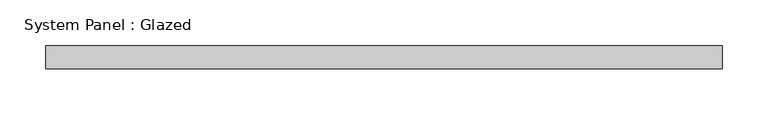
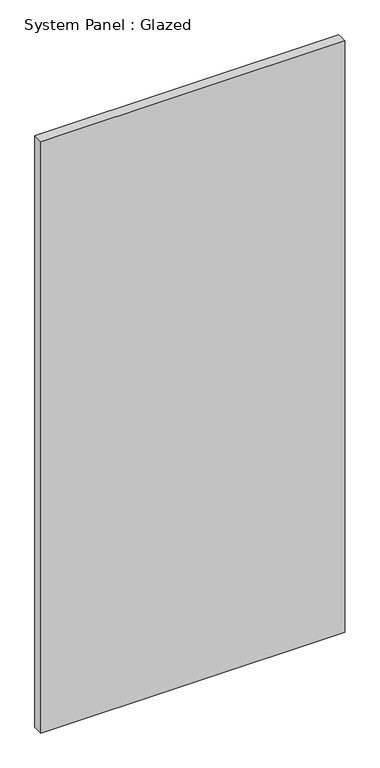
"""IFC4 building model written with IfcOpenShell, lengths in millimetres: plate geometry, System Panel : Glazed."""

from ifc_helpers import new_model, si_unit, origin, origin_with_axes, place, context, project, spatial, polyline, outline, extrude, source, transform, mapped, element, save


def system_panel_glazed_3e14b5a9(model_context):
    return source(origin(), model_context, "Body", "SweptSolid", [
        extrude(outline(polyline([(370.1056477, 19.05), (-370.1056477, 19.05), (-370.1056477, 44.45), (370.1056477, 44.45), (370.1056477, 19.05)])), origin_with_axes(), (0.0, 0.0, 1.0), 1522.9537661),
    ])


if __name__ == "__main__":
    model = new_model("IFC4")
    model_context = context("Model", 3, world=origin())
    ifc_project = project(units=[si_unit("LENGTHUNIT", "METRE", prefix="MILLI")], contexts=[model_context])
    site = spatial("IfcSite", under=ifc_project)
    building = spatial("IfcBuilding", under=site)
    placement = place(None, origin())
    system_panel_glazed_shape = system_panel_glazed_3e14b5a9(model_context)
    element("IfcPlate", 1, ObjectType="System Panel : Glazed", at=placement, inside=building, context=model_context, shape_type="MappedRepresentation", body=[
        mapped(system_panel_glazed_shape, transform((0.0, 0.0, 0.0), x_axis=(1.0, 0.0, 0.0), y_axis=(0.0, 1.0, 0.0), z_axis=(0.0, 0.0, 1.0))),
    ])
    save(model, "model.ifc")

# Revit data of these elements
# Type "System Panel : Glazed"
#   Construction Type Id = "GSP4R"
#   Analytic Construction = "1/8 in Pilkington single glazing"
#   Visual Light Transmittance = 0.9
#   Solar Heat Gain Coefficient = 0.86
#   Heat Transfer Coefficient (U) = 1.18115 BTU/(h·ft²·°F)
#   Define Thermal Properties by = 1
# Element 1 (IfcPlate, "System Panel : Glazed")
#   Materials on its faces: "Glass"
# Materials
#   "Glass": class "Glass", colour RGB 0 128 192, transparency 0.75, Description = "Soda Lime Glass", Cost = 0
